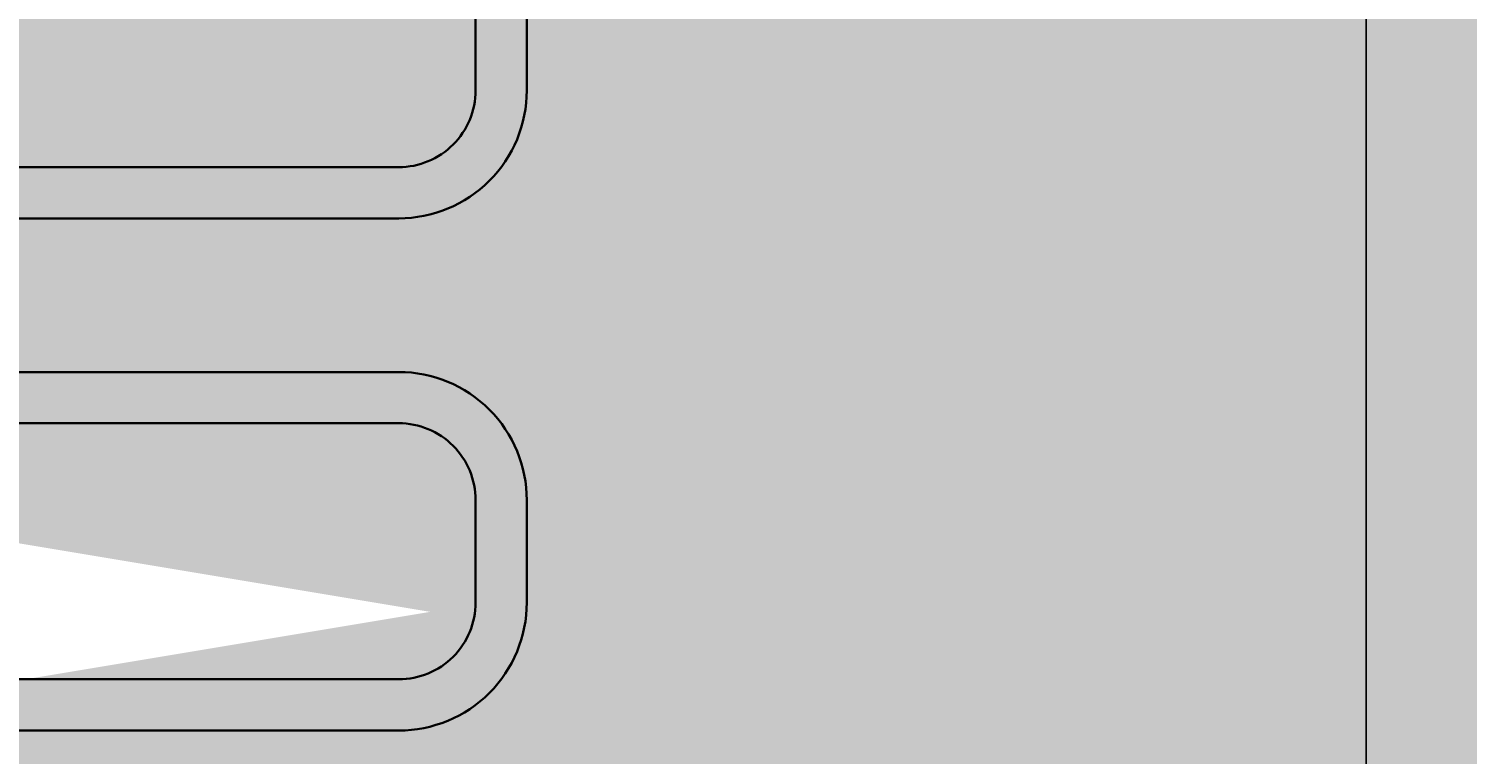
# Model space of a CAD drawing. Units: millimetres. Extents: x -22994 to 29398, y -19990 to 20176.
# Tile 48 of 135: x 170 to 198, y 96 to 110. Entities that reach past the tile are written whole.
import ezdxf

# ---------------------------------------------------------------- set-up
doc = ezdxf.new("R2010")
doc.units = ezdxf.units.MM
doc.header["$MEASUREMENT"] = 0
for name, color, linetype, lineweight in [('M-DIMS', 2, 'Continuous', 18), ('M-EQPM', 7, 'Continuous', 25), ('M-EQPM-PATT', 7, 'Continuous', 18), ('M-PIPE', 7, 'Continuous', 35)]:
    doc.layers.add(name, color=color, linetype=linetype, lineweight=lineweight)
doc.styles.get("Standard").update_dxf_attribs({"font": 'arial.ttf'})
doc.dimstyles.get("Standard").update_dxf_attribs({"dimtxt": 0.18, "dimasz": 10000, "dimexe": 0.18, "dimexo": 0.0625, "dimgap": 0.09, "dimtad": 0, "dimtih": 1, "dimtoh": 1, "dimdec": 0, "dimzin": 0, "dimdsep": 46, "dimtxsty": 'Standard', "dimcen": 0.09, "dimadec": 0, "dimazin": 0, "dimtfac": 1, "dimtdec": 0, "dimtofl": 0, "dimtmove": 0, "dimatfit": 3, "dimfxl": 1, "dimtolj": 1, "dimtzin": 0, "dimlwd": 30, "dimarcsym": 0})

# ---------------------------------------------------------------- blocks, each defined once
blk = doc.blocks.new('*D2')
at = {"layer": 'Defpoints', "color": 0, "transparency": 16777216}
for p in [(6.677, 10.271), (290.852, 10.271), (290.852, -5.079)]:
    blk.add_point(p, dxfattribs=at)
at = {"layer": 'M-DIMS', "color": 0, "lineweight": -2, "transparency": 16777216}
for p, q in [((6.677, 10.209), (6.677, -5.259)), ((290.852, 10.209), (290.852, -5.259))]:
    blk.add_line(p, q, dxfattribs=at)
at = {"layer": 'M-DIMS', "color": 0, "lineweight": 30, "transparency": 16777216}
for p, q in [((-9993.323, -5.079), (-19993.323, -5.079)), ((10290.852, -5.079), (20290.852, -5.079))]:
    blk.add_line(p, q, dxfattribs=at)
at = {"layer": 'M-DIMS', "color": 0, "transparency": 16777216}
for points in [[(-9993.323, 1661.588), (-9993.323, -1671.745), (6.677, -5.079)], [(10290.852, 1661.588), (10290.852, -1671.745), (290.852, -5.079)]]:
    blk.add_solid(points, dxfattribs=at)
at = {"layer": 'M-DIMS', "color": 0, "transparency": 16777216, "insert": (148.765, -5.079), "char_height": 0.18, "attachment_point": 5}
blk.add_mtext('\\A1;284.2', dxfattribs=at)
blk = doc.blocks.new('*D3')
at = {"layer": 'Defpoints', "color": 0, "transparency": 16777216}
for p in [(110.265, 204.165), (110.265, 176.366), (95.833, 127.967)]:
    blk.add_point(p, dxfattribs=at)
at = {"layer": 'M-DIMS', "color": 0, "lineweight": 30, "transparency": 16777216}
for p, q in [((-9904.167, 204.165), (-19904.167, 204.165)), ((10110.265, 204.165), (20110.265, 204.165))]:
    blk.add_line(p, q, dxfattribs=at)
at = {"layer": 'M-DIMS', "color": 0, "lineweight": -2, "transparency": 16777216}
for p, q in [((95.833, 128.03), (95.833, 204.345)), ((110.265, 176.429), (110.265, 204.345))]:
    blk.add_line(p, q, dxfattribs=at)
at = {"layer": 'M-DIMS', "color": 0, "transparency": 16777216}
for points in [[(-9904.167, 1870.832), (-9904.167, -1462.501), (95.833, 204.165)], [(10110.265, 1870.832), (10110.265, -1462.501), (110.265, 204.165)]]:
    blk.add_solid(points, dxfattribs=at)
at = {"layer": 'M-DIMS', "color": 0, "transparency": 16777216, "insert": (103.049, 204.165), "char_height": 0.18, "attachment_point": 5}
blk.add_mtext('\\A1;14.432', dxfattribs=at)
blk = doc.blocks.new('*D4')
at = {"layer": 'Defpoints', "color": 0, "transparency": 16777216}
for p in [(116.265, 204.165), (110.265, 176.366), (116.265, 176.366)]:
    blk.add_point(p, dxfattribs=at)
at = {"layer": 'M-DIMS', "color": 0, "lineweight": 30, "transparency": 16777216}
for p, q in [((-9889.735, 204.165), (-19889.735, 204.165)), ((10116.265, 204.165), (20116.265, 204.165))]:
    blk.add_line(p, q, dxfattribs=at)
at = {"layer": 'M-DIMS', "color": 0, "lineweight": -2, "transparency": 16777216}
for p, q in [((110.265, 176.429), (110.265, 204.345)), ((116.265, 176.429), (116.265, 204.345))]:
    blk.add_line(p, q, dxfattribs=at)
at = {"layer": 'M-DIMS', "color": 0, "transparency": 16777216}
for points in [[(-9889.735, 1870.832), (-9889.735, -1462.501), (110.265, 204.165)], [(10116.265, 1870.832), (10116.265, -1462.501), (116.265, 204.165)]]:
    blk.add_solid(points, dxfattribs=at)
at = {"layer": 'M-DIMS', "color": 0, "transparency": 16777216, "insert": (113.265, 204.165), "char_height": 0.18, "attachment_point": 5}
blk.add_mtext('\\A1;6', dxfattribs=at)
blk = doc.blocks.new('*D5')
at = {"layer": 'Defpoints', "color": 0, "transparency": 16777216}
for p in [(181.265, 204.165), (116.265, 176.366), (181.265, 176.366)]:
    blk.add_point(p, dxfattribs=at)
at = {"layer": 'M-DIMS', "color": 0, "lineweight": 30, "transparency": 16777216}
for p, q in [((-9883.735, 204.165), (-19883.735, 204.165)), ((10181.265, 204.165), (20181.265, 204.165))]:
    blk.add_line(p, q, dxfattribs=at)
at = {"layer": 'M-DIMS', "color": 0, "lineweight": -2, "transparency": 16777216}
for p, q in [((116.265, 176.429), (116.265, 204.345)), ((181.265, 176.429), (181.265, 204.345))]:
    blk.add_line(p, q, dxfattribs=at)
at = {"layer": 'M-DIMS', "color": 0, "transparency": 16777216}
for points in [[(-9883.735, 1870.832), (-9883.735, -1462.501), (116.265, 204.165)], [(10181.265, 1870.832), (10181.265, -1462.501), (181.265, 204.165)]]:
    blk.add_solid(points, dxfattribs=at)
at = {"layer": 'M-DIMS', "color": 0, "transparency": 16777216, "insert": (148.765, 204.165), "char_height": 0.18, "attachment_point": 5}
blk.add_mtext('\\A1;65', dxfattribs=at)
blk = doc.blocks.new('*D6')
at = {"layer": 'Defpoints', "color": 0, "transparency": 16777216}
for p in [(187.265, 204.165), (181.265, 176.366), (187.265, 176.366)]:
    blk.add_point(p, dxfattribs=at)
at = {"layer": 'M-DIMS', "color": 0, "lineweight": 30, "transparency": 16777216}
for p, q in [((-9818.735, 204.165), (-19818.735, 204.165)), ((10187.265, 204.165), (20187.265, 204.165))]:
    blk.add_line(p, q, dxfattribs=at)
at = {"layer": 'M-DIMS', "color": 0, "lineweight": -2, "transparency": 16777216}
for p, q in [((181.265, 176.429), (181.265, 204.345)), ((187.265, 176.429), (187.265, 204.345))]:
    blk.add_line(p, q, dxfattribs=at)
at = {"layer": 'M-DIMS', "color": 0, "transparency": 16777216}
for points in [[(-9818.735, 1870.832), (-9818.735, -1462.501), (181.265, 204.165)], [(10187.265, 1870.832), (10187.265, -1462.501), (187.265, 204.165)]]:
    blk.add_solid(points, dxfattribs=at)
at = {"layer": 'M-DIMS', "color": 0, "transparency": 16777216, "insert": (184.265, 204.165), "char_height": 0.18, "attachment_point": 5}
blk.add_mtext('\\A1;6', dxfattribs=at)
blk = doc.blocks.new('*D7')
at = {"layer": 'Defpoints', "color": 0, "transparency": 16777216}
for p in [(201.697, 204.165), (187.265, 176.366), (201.697, 127.967)]:
    blk.add_point(p, dxfattribs=at)
at = {"layer": 'M-DIMS', "color": 0, "lineweight": 30, "transparency": 16777216}
for p, q in [((-9812.735, 204.165), (-19812.735, 204.165)), ((10201.697, 204.165), (20201.697, 204.165))]:
    blk.add_line(p, q, dxfattribs=at)
at = {"layer": 'M-DIMS', "color": 0, "lineweight": -2, "transparency": 16777216}
for p, q in [((187.265, 176.429), (187.265, 204.345)), ((201.697, 128.03), (201.697, 204.345))]:
    blk.add_line(p, q, dxfattribs=at)
at = {"layer": 'M-DIMS', "color": 0, "transparency": 16777216}
for points in [[(-9812.735, 1870.832), (-9812.735, -1462.501), (187.265, 204.165)], [(10201.697, 1870.832), (10201.697, -1462.501), (201.697, 204.165)]]:
    blk.add_solid(points, dxfattribs=at)
at = {"layer": 'M-DIMS', "color": 0, "transparency": 16777216, "insert": (194.481, 204.165), "char_height": 0.18, "attachment_point": 5}
blk.add_mtext('\\A1;14.432', dxfattribs=at)
blk = doc.blocks.new('*D8')
at = {"layer": 'Defpoints', "color": 0, "transparency": 16777216}
for p in [(227.648, 204.165), (227.648, 146.73), (201.697, 127.967)]:
    blk.add_point(p, dxfattribs=at)
at = {"layer": 'M-DIMS', "color": 0, "lineweight": 30, "transparency": 16777216}
for p, q in [((-9798.303, 204.165), (-19798.303, 204.165)), ((10227.648, 204.165), (20227.648, 204.165))]:
    blk.add_line(p, q, dxfattribs=at)
at = {"layer": 'M-DIMS', "color": 0, "lineweight": -2, "transparency": 16777216}
for p, q in [((201.697, 128.03), (201.697, 204.345)), ((227.648, 146.792), (227.648, 204.345))]:
    blk.add_line(p, q, dxfattribs=at)
at = {"layer": 'M-DIMS', "color": 0, "transparency": 16777216}
for points in [[(-9798.303, 1870.832), (-9798.303, -1462.501), (201.697, 204.165)], [(10227.648, 1870.832), (10227.648, -1462.501), (227.648, 204.165)]]:
    blk.add_solid(points, dxfattribs=at)
at = {"layer": 'M-DIMS', "color": 0, "transparency": 16777216, "insert": (214.673, 204.165), "char_height": 0.18, "attachment_point": 5}
blk.add_mtext('\\A1;25.95', dxfattribs=at)
blk = doc.blocks.new('*D9')
at = {"layer": 'Defpoints', "color": 0, "transparency": 16777216}
for p in [(187.265, 176.366), (306.202, 176.366), (290.852, 10.271)]:
    blk.add_point(p, dxfattribs=at)
at = {"layer": 'M-DIMS', "color": 0, "lineweight": 30, "transparency": 16777216}
for p, q in [((306.202, 10176.366), (306.202, 20176.366)), ((306.202, -9989.729), (306.202, -19989.729))]:
    blk.add_line(p, q, dxfattribs=at)
at = {"layer": 'M-DIMS', "color": 0, "lineweight": -2, "transparency": 16777216}
for p, q in [((187.327, 176.366), (306.382, 176.366)), ((290.915, 10.271), (306.382, 10.271))]:
    blk.add_line(p, q, dxfattribs=at)
at = {"layer": 'M-DIMS', "color": 0, "transparency": 16777216}
for points in [[(-1360.465, 10176.366), (1972.869, 10176.366), (306.202, 176.366)], [(-1360.465, -9989.729), (1972.869, -9989.729), (306.202, 10.271)]]:
    blk.add_solid(points, dxfattribs=at)
at = {"layer": 'M-DIMS', "color": 0, "transparency": 16777216, "insert": (306.202, 93.319), "char_height": 0.18, "attachment_point": 5}
blk.add_mtext('\\A1;166.1', dxfattribs=at)
blk = doc.blocks.new('*D10')
at = {"layer": 'Defpoints', "color": 0, "transparency": 16777216}
for p in [(125.65, 136.071), (133.346, 136.071), (133.346, -5.079)]:
    blk.add_point(p, dxfattribs=at)
at = {"layer": 'M-DIMS', "color": 0, "lineweight": -2, "transparency": 16777216}
for p, q in [((125.65, 136.009), (125.65, -5.259)), ((133.346, 136.009), (133.346, -5.259))]:
    blk.add_line(p, q, dxfattribs=at)
at = {"layer": 'M-DIMS', "color": 0, "lineweight": 30, "transparency": 16777216}
for p, q in [((-9874.35, -5.079), (-19874.35, -5.079)), ((10133.346, -5.079), (20133.346, -5.079))]:
    blk.add_line(p, q, dxfattribs=at)
at = {"layer": 'M-DIMS', "color": 0, "transparency": 16777216}
for points in [[(-9874.35, 1661.588), (-9874.35, -1671.745), (125.65, -5.079)], [(10133.346, 1661.588), (10133.346, -1671.745), (133.346, -5.079)]]:
    blk.add_solid(points, dxfattribs=at)
at = {"layer": 'M-DIMS', "color": 0, "transparency": 16777216, "insert": (129.498, -5.079), "char_height": 0.18, "attachment_point": 5}
blk.add_mtext('\\A1;7.696', dxfattribs=at)
blk = doc.blocks.new('*D11')
at = {"layer": 'Defpoints', "color": 0, "transparency": 16777216}
for p in [(133.346, 136.071), (135.65, 136.071), (135.65, -5.079)]:
    blk.add_point(p, dxfattribs=at)
at = {"layer": 'M-DIMS', "color": 0, "lineweight": -2, "transparency": 16777216}
for p, q in [((133.346, 136.009), (133.346, -5.259)), ((135.65, 136.009), (135.65, -5.259))]:
    blk.add_line(p, q, dxfattribs=at)
at = {"layer": 'M-DIMS', "color": 0, "lineweight": 30, "transparency": 16777216}
for p, q in [((-9866.654, -5.079), (-19866.654, -5.079)), ((10135.65, -5.079), (20135.65, -5.079))]:
    blk.add_line(p, q, dxfattribs=at)
at = {"layer": 'M-DIMS', "color": 0, "transparency": 16777216}
for points in [[(-9866.654, 1661.588), (-9866.654, -1671.745), (133.346, -5.079)], [(10135.65, 1661.588), (10135.65, -1671.745), (135.65, -5.079)]]:
    blk.add_solid(points, dxfattribs=at)
at = {"layer": 'M-DIMS', "color": 0, "transparency": 16777216, "insert": (134.498, -5.079), "char_height": 0.18, "attachment_point": 5}
blk.add_mtext('\\A1;2.304', dxfattribs=at)
blk = doc.blocks.new('*D12')
at = {"layer": 'Defpoints', "color": 0, "transparency": 16777216}
for p in [(135.65, 136.071), (145.65, 136.071), (145.65, -5.079)]:
    blk.add_point(p, dxfattribs=at)
at = {"layer": 'M-DIMS', "color": 0, "lineweight": -2, "transparency": 16777216}
for p, q in [((135.65, 136.009), (135.65, -5.259)), ((145.65, 136.009), (145.65, -5.259))]:
    blk.add_line(p, q, dxfattribs=at)
at = {"layer": 'M-DIMS', "color": 0, "lineweight": 30, "transparency": 16777216}
for p, q in [((-9864.35, -5.079), (-19864.35, -5.079)), ((10145.65, -5.079), (20145.65, -5.079))]:
    blk.add_line(p, q, dxfattribs=at)
at = {"layer": 'M-DIMS', "color": 0, "transparency": 16777216}
for points in [[(-9864.35, 1661.588), (-9864.35, -1671.745), (135.65, -5.079)], [(10145.65, 1661.588), (10145.65, -1671.745), (145.65, -5.079)]]:
    blk.add_solid(points, dxfattribs=at)
at = {"layer": 'M-DIMS', "color": 0, "transparency": 16777216, "insert": (140.65, -5.079), "char_height": 0.18, "attachment_point": 5}
blk.add_mtext('\\A1;10', dxfattribs=at)
blk = doc.blocks.new('*D13')
at = {"layer": 'Defpoints', "color": 0, "transparency": 16777216}
for p in [(145.65, 136.071), (155.65, 136.071), (155.65, -5.079)]:
    blk.add_point(p, dxfattribs=at)
at = {"layer": 'M-DIMS', "color": 0, "lineweight": -2, "transparency": 16777216}
for p, q in [((145.65, 136.009), (145.65, -5.259)), ((155.65, 136.009), (155.65, -5.259))]:
    blk.add_line(p, q, dxfattribs=at)
at = {"layer": 'M-DIMS', "color": 0, "lineweight": 30, "transparency": 16777216}
for p, q in [((-9854.35, -5.079), (-19854.35, -5.079)), ((10155.65, -5.079), (20155.65, -5.079))]:
    blk.add_line(p, q, dxfattribs=at)
at = {"layer": 'M-DIMS', "color": 0, "transparency": 16777216}
for points in [[(-9854.35, 1661.588), (-9854.35, -1671.745), (145.65, -5.079)], [(10155.65, 1661.588), (10155.65, -1671.745), (155.65, -5.079)]]:
    blk.add_solid(points, dxfattribs=at)
at = {"layer": 'M-DIMS', "color": 0, "transparency": 16777216, "insert": (150.65, -5.079), "char_height": 0.18, "attachment_point": 5}
blk.add_mtext('\\A1;10', dxfattribs=at)
blk = doc.blocks.new('*D14')
at = {"layer": 'Defpoints', "color": 0, "transparency": 16777216}
for p in [(155.65, 136.071), (165.65, 136.071), (165.65, -5.079)]:
    blk.add_point(p, dxfattribs=at)
at = {"layer": 'M-DIMS', "color": 0, "lineweight": -2, "transparency": 16777216}
for p, q in [((155.65, 136.009), (155.65, -5.259)), ((165.65, 136.009), (165.65, -5.259))]:
    blk.add_line(p, q, dxfattribs=at)
at = {"layer": 'M-DIMS', "color": 0, "lineweight": 30, "transparency": 16777216}
for p, q in [((-9844.35, -5.079), (-19844.35, -5.079)), ((10165.65, -5.079), (20165.65, -5.079))]:
    blk.add_line(p, q, dxfattribs=at)
at = {"layer": 'M-DIMS', "color": 0, "transparency": 16777216}
for points in [[(-9844.35, 1661.588), (-9844.35, -1671.745), (155.65, -5.079)], [(10165.65, 1661.588), (10165.65, -1671.745), (165.65, -5.079)]]:
    blk.add_solid(points, dxfattribs=at)
at = {"layer": 'M-DIMS', "color": 0, "transparency": 16777216, "insert": (160.65, -5.079), "char_height": 0.18, "attachment_point": 5}
blk.add_mtext('\\A1;10', dxfattribs=at)
blk = doc.blocks.new('*D15')
at = {"layer": 'Defpoints', "color": 0, "transparency": 16777216}
for p in [(173.346, 154.788), (173.346, 136.071), (306.202, 136.071)]:
    blk.add_point(p, dxfattribs=at)
at = {"layer": 'M-DIMS', "color": 0, "lineweight": 30, "transparency": 16777216}
for p, q in [((306.202, 10154.788), (306.202, 20154.788)), ((306.202, -9863.929), (306.202, -19863.929))]:
    blk.add_line(p, q, dxfattribs=at)
at = {"layer": 'M-DIMS', "color": 0, "lineweight": -2, "transparency": 16777216}
for p, q in [((173.408, 154.788), (306.382, 154.788)), ((173.408, 136.071), (306.382, 136.071))]:
    blk.add_line(p, q, dxfattribs=at)
at = {"layer": 'M-DIMS', "color": 0, "transparency": 16777216}
for points in [[(-1360.465, 10154.788), (1972.869, 10154.788), (306.202, 154.788)], [(-1360.465, -9863.929), (1972.869, -9863.929), (306.202, 136.071)]]:
    blk.add_solid(points, dxfattribs=at)
at = {"layer": 'M-DIMS', "color": 0, "transparency": 16777216, "insert": (306.202, 145.43), "char_height": 0.18, "attachment_point": 5}
blk.add_mtext('\\A1;18.717', dxfattribs=at)
blk = doc.blocks.new('*D16')
at = {"layer": 'Defpoints', "color": 0, "transparency": 16777216}
for p in [(120.17, 204.165), (110.466, 48.035), (120.17, 48.035)]:
    blk.add_point(p, dxfattribs=at)
at = {"layer": 'M-DIMS', "color": 0, "lineweight": 30, "transparency": 16777216}
for p, q in [((-9889.534, 204.165), (-19889.534, 204.165)), ((10120.17, 204.165), (20120.17, 204.165))]:
    blk.add_line(p, q, dxfattribs=at)
at = {"layer": 'M-DIMS', "color": 0, "lineweight": -2, "transparency": 16777216}
for p, q in [((110.466, 48.097), (110.466, 204.345)), ((120.17, 48.097), (120.17, 204.345))]:
    blk.add_line(p, q, dxfattribs=at)
at = {"layer": 'M-DIMS', "color": 0, "transparency": 16777216}
for points in [[(-9889.534, 1870.832), (-9889.534, -1462.501), (110.466, 204.165)], [(10120.17, 1870.832), (10120.17, -1462.501), (120.17, 204.165)]]:
    blk.add_solid(points, dxfattribs=at)
at = {"layer": 'M-DIMS', "color": 0, "transparency": 16777216, "insert": (115.318, 204.165), "char_height": 0.18, "attachment_point": 5}
blk.add_mtext('\\A1;9.704', dxfattribs=at)
blk = doc.blocks.new('*D17')
at = {"layer": 'Defpoints', "color": 0, "transparency": 16777216}
for p in [(126.17, 204.165), (120.17, 48.035), (126.17, 48.035)]:
    blk.add_point(p, dxfattribs=at)
at = {"layer": 'M-DIMS', "color": 0, "lineweight": 30, "transparency": 16777216}
for p, q in [((-9879.83, 204.165), (-19879.83, 204.165)), ((10126.17, 204.165), (20126.17, 204.165))]:
    blk.add_line(p, q, dxfattribs=at)
at = {"layer": 'M-DIMS', "color": 0, "lineweight": -2, "transparency": 16777216}
for p, q in [((120.17, 48.097), (120.17, 204.345)), ((126.17, 48.097), (126.17, 204.345))]:
    blk.add_line(p, q, dxfattribs=at)
at = {"layer": 'M-DIMS', "color": 0, "transparency": 16777216}
for points in [[(-9879.83, 1870.832), (-9879.83, -1462.501), (120.17, 204.165)], [(10126.17, 1870.832), (10126.17, -1462.501), (126.17, 204.165)]]:
    blk.add_solid(points, dxfattribs=at)
at = {"layer": 'M-DIMS', "color": 0, "transparency": 16777216, "insert": (123.17, 204.165), "char_height": 0.18, "attachment_point": 5}
blk.add_mtext('\\A1;6', dxfattribs=at)
blk = doc.blocks.new('*D18')
at = {"layer": 'Defpoints', "color": 0, "transparency": 16777216}
for p in [(132.17, 204.165), (126.17, 48.035), (132.17, 48.035)]:
    blk.add_point(p, dxfattribs=at)
at = {"layer": 'M-DIMS', "color": 0, "lineweight": 30, "transparency": 16777216}
for p, q in [((-9873.83, 204.165), (-19873.83, 204.165)), ((10132.17, 204.165), (20132.17, 204.165))]:
    blk.add_line(p, q, dxfattribs=at)
at = {"layer": 'M-DIMS', "color": 0, "lineweight": -2, "transparency": 16777216}
for p, q in [((126.17, 48.097), (126.17, 204.345)), ((132.17, 48.097), (132.17, 204.345))]:
    blk.add_line(p, q, dxfattribs=at)
at = {"layer": 'M-DIMS', "color": 0, "transparency": 16777216}
for points in [[(-9873.83, 1870.832), (-9873.83, -1462.501), (126.17, 204.165)], [(10132.17, 1870.832), (10132.17, -1462.501), (132.17, 204.165)]]:
    blk.add_solid(points, dxfattribs=at)
at = {"layer": 'M-DIMS', "color": 0, "transparency": 16777216, "insert": (129.17, 204.165), "char_height": 0.18, "attachment_point": 5}
blk.add_mtext('\\A1;6', dxfattribs=at)
blk = doc.blocks.new('*D19')
at = {"layer": 'Defpoints', "color": 0, "transparency": 16777216}
for p in [(138.17, 204.165), (132.17, 48.035), (138.17, 48.035)]:
    blk.add_point(p, dxfattribs=at)
at = {"layer": 'M-DIMS', "color": 0, "lineweight": 30, "transparency": 16777216}
for p, q in [((-9867.83, 204.165), (-19867.83, 204.165)), ((10138.17, 204.165), (20138.17, 204.165))]:
    blk.add_line(p, q, dxfattribs=at)
at = {"layer": 'M-DIMS', "color": 0, "lineweight": -2, "transparency": 16777216}
for p, q in [((132.17, 48.097), (132.17, 204.345)), ((138.17, 48.097), (138.17, 204.345))]:
    blk.add_line(p, q, dxfattribs=at)
at = {"layer": 'M-DIMS', "color": 0, "transparency": 16777216}
for points in [[(-9867.83, 1870.832), (-9867.83, -1462.501), (132.17, 204.165)], [(10138.17, 1870.832), (10138.17, -1462.501), (138.17, 204.165)]]:
    blk.add_solid(points, dxfattribs=at)
at = {"layer": 'M-DIMS', "color": 0, "transparency": 16777216, "insert": (135.17, 204.165), "char_height": 0.18, "attachment_point": 5}
blk.add_mtext('\\A1;6', dxfattribs=at)
blk = doc.blocks.new('*D20')
at = {"layer": 'Defpoints', "color": 0, "transparency": 16777216}
for p in [(144.17, 204.165), (138.17, 48.035), (144.17, 48.035)]:
    blk.add_point(p, dxfattribs=at)
at = {"layer": 'M-DIMS', "color": 0, "lineweight": 30, "transparency": 16777216}
for p, q in [((-9861.83, 204.165), (-19861.83, 204.165)), ((10144.17, 204.165), (20144.17, 204.165))]:
    blk.add_line(p, q, dxfattribs=at)
at = {"layer": 'M-DIMS', "color": 0, "lineweight": -2, "transparency": 16777216}
for p, q in [((138.17, 48.097), (138.17, 204.345)), ((144.17, 48.097), (144.17, 204.345))]:
    blk.add_line(p, q, dxfattribs=at)
at = {"layer": 'M-DIMS', "color": 0, "transparency": 16777216}
for points in [[(-9861.83, 1870.832), (-9861.83, -1462.501), (138.17, 204.165)], [(10144.17, 1870.832), (10144.17, -1462.501), (144.17, 204.165)]]:
    blk.add_solid(points, dxfattribs=at)
at = {"layer": 'M-DIMS', "color": 0, "transparency": 16777216, "insert": (141.17, 204.165), "char_height": 0.18, "attachment_point": 5}
blk.add_mtext('\\A1;6', dxfattribs=at)
blk = doc.blocks.new('*D21')
at = {"layer": 'Defpoints', "color": 0, "transparency": 16777216}
for p in [(149.116, 204.165), (144.17, 48.035), (149.116, 48.035)]:
    blk.add_point(p, dxfattribs=at)
at = {"layer": 'M-DIMS', "color": 0, "lineweight": 30, "transparency": 16777216}
for p, q in [((-9855.83, 204.165), (-19855.83, 204.165)), ((10149.116, 204.165), (20149.116, 204.165))]:
    blk.add_line(p, q, dxfattribs=at)
at = {"layer": 'M-DIMS', "color": 0, "lineweight": -2, "transparency": 16777216}
for p, q in [((144.17, 48.097), (144.17, 204.345)), ((149.116, 48.097), (149.116, 204.345))]:
    blk.add_line(p, q, dxfattribs=at)
at = {"layer": 'M-DIMS', "color": 0, "transparency": 16777216}
for points in [[(-9855.83, 1870.832), (-9855.83, -1462.501), (144.17, 204.165)], [(10149.116, 1870.832), (10149.116, -1462.501), (149.116, 204.165)]]:
    blk.add_solid(points, dxfattribs=at)
at = {"layer": 'M-DIMS', "color": 0, "transparency": 16777216, "insert": (146.643, 204.165), "char_height": 0.18, "attachment_point": 5}
blk.add_mtext('\\A1;4.945', dxfattribs=at)
blk = doc.blocks.new('*D22')
at = {"layer": 'Defpoints', "color": 0, "transparency": 16777216}
for p in [(149.116, 30.99), (155.116, 30.99), (155.116, -5.079)]:
    blk.add_point(p, dxfattribs=at)
at = {"layer": 'M-DIMS', "color": 0, "lineweight": -2, "transparency": 16777216}
for p, q in [((149.116, 30.927), (149.116, -5.259)), ((155.116, 30.927), (155.116, -5.259))]:
    blk.add_line(p, q, dxfattribs=at)
at = {"layer": 'M-DIMS', "color": 0, "lineweight": 30, "transparency": 16777216}
for p, q in [((-9850.884, -5.079), (-19850.884, -5.079)), ((10155.116, -5.079), (20155.116, -5.079))]:
    blk.add_line(p, q, dxfattribs=at)
at = {"layer": 'M-DIMS', "color": 0, "transparency": 16777216}
for points in [[(-9850.884, 1661.588), (-9850.884, -1671.745), (149.116, -5.079)], [(10155.116, 1661.588), (10155.116, -1671.745), (155.116, -5.079)]]:
    blk.add_solid(points, dxfattribs=at)
at = {"layer": 'M-DIMS', "color": 0, "transparency": 16777216, "insert": (152.116, -5.079), "char_height": 0.18, "attachment_point": 5}
blk.add_mtext('\\A1;6', dxfattribs=at)
blk = doc.blocks.new('*D23')
at = {"layer": 'Defpoints', "color": 0, "transparency": 16777216}
for p in [(155.116, 30.99), (161.116, 30.99), (161.116, -5.079)]:
    blk.add_point(p, dxfattribs=at)
at = {"layer": 'M-DIMS', "color": 0, "lineweight": -2, "transparency": 16777216}
for p, q in [((155.116, 30.927), (155.116, -5.259)), ((161.116, 30.927), (161.116, -5.259))]:
    blk.add_line(p, q, dxfattribs=at)
at = {"layer": 'M-DIMS', "color": 0, "lineweight": 30, "transparency": 16777216}
for p, q in [((-9844.884, -5.079), (-19844.884, -5.079)), ((10161.116, -5.079), (20161.116, -5.079))]:
    blk.add_line(p, q, dxfattribs=at)
at = {"layer": 'M-DIMS', "color": 0, "transparency": 16777216}
for points in [[(-9844.884, 1661.588), (-9844.884, -1671.745), (155.116, -5.079)], [(10161.116, 1661.588), (10161.116, -1671.745), (161.116, -5.079)]]:
    blk.add_solid(points, dxfattribs=at)
at = {"layer": 'M-DIMS', "color": 0, "transparency": 16777216, "insert": (158.116, -5.079), "char_height": 0.18, "attachment_point": 5}
blk.add_mtext('\\A1;6', dxfattribs=at)
blk = doc.blocks.new('*D24')
at = {"layer": 'Defpoints', "color": 0, "transparency": 16777216}
for p in [(161.116, 30.99), (166.439, 30.99), (166.439, -5.079)]:
    blk.add_point(p, dxfattribs=at)
at = {"layer": 'M-DIMS', "color": 0, "lineweight": -2, "transparency": 16777216}
for p, q in [((161.116, 30.927), (161.116, -5.259)), ((166.439, 30.927), (166.439, -5.259))]:
    blk.add_line(p, q, dxfattribs=at)
at = {"layer": 'M-DIMS', "color": 0, "lineweight": 30, "transparency": 16777216}
for p, q in [((-9838.884, -5.079), (-19838.884, -5.079)), ((10166.439, -5.079), (20166.439, -5.079))]:
    blk.add_line(p, q, dxfattribs=at)
at = {"layer": 'M-DIMS', "color": 0, "transparency": 16777216}
for points in [[(-9838.884, 1661.588), (-9838.884, -1671.745), (161.116, -5.079)], [(10166.439, 1661.588), (10166.439, -1671.745), (166.439, -5.079)]]:
    blk.add_solid(points, dxfattribs=at)
at = {"layer": 'M-DIMS', "color": 0, "transparency": 16777216, "insert": (163.777, -5.079), "char_height": 0.18, "attachment_point": 5}
blk.add_mtext('\\A1;5.323', dxfattribs=at)
blk = doc.blocks.new('*D25')
at = {"layer": 'Defpoints', "color": 0, "transparency": 16777216}
for p in [(166.439, 30.99), (172.439, 30.99), (172.439, -5.079)]:
    blk.add_point(p, dxfattribs=at)
at = {"layer": 'M-DIMS', "color": 0, "lineweight": -2, "transparency": 16777216}
for p, q in [((166.439, 30.927), (166.439, -5.259)), ((172.439, 30.927), (172.439, -5.259))]:
    blk.add_line(p, q, dxfattribs=at)
at = {"layer": 'M-DIMS', "color": 0, "lineweight": 30, "transparency": 16777216}
for p, q in [((-9833.561, -5.079), (-19833.561, -5.079)), ((10172.439, -5.079), (20172.439, -5.079))]:
    blk.add_line(p, q, dxfattribs=at)
at = {"layer": 'M-DIMS', "color": 0, "transparency": 16777216}
for points in [[(-9833.561, 1661.588), (-9833.561, -1671.745), (166.439, -5.079)], [(10172.439, 1661.588), (10172.439, -1671.745), (172.439, -5.079)]]:
    blk.add_solid(points, dxfattribs=at)
at = {"layer": 'M-DIMS', "color": 0, "transparency": 16777216, "insert": (169.439, -5.079), "char_height": 0.18, "attachment_point": 5}
blk.add_mtext('\\A1;6', dxfattribs=at)
blk = doc.blocks.new('*D26')
at = {"layer": 'Defpoints', "color": 0, "transparency": 16777216}
for p in [(172.439, 30.99), (178.439, 30.99), (178.439, -5.079)]:
    blk.add_point(p, dxfattribs=at)
at = {"layer": 'M-DIMS', "color": 0, "lineweight": -2, "transparency": 16777216}
for p, q in [((172.439, 30.927), (172.439, -5.259)), ((178.439, 30.927), (178.439, -5.259))]:
    blk.add_line(p, q, dxfattribs=at)
at = {"layer": 'M-DIMS', "color": 0, "lineweight": 30, "transparency": 16777216}
for p, q in [((-9827.561, -5.079), (-19827.561, -5.079)), ((10178.439, -5.079), (20178.439, -5.079))]:
    blk.add_line(p, q, dxfattribs=at)
at = {"layer": 'M-DIMS', "color": 0, "transparency": 16777216}
for points in [[(-9827.561, 1661.588), (-9827.561, -1671.745), (172.439, -5.079)], [(10178.439, 1661.588), (10178.439, -1671.745), (178.439, -5.079)]]:
    blk.add_solid(points, dxfattribs=at)
at = {"layer": 'M-DIMS', "color": 0, "transparency": 16777216, "insert": (175.439, -5.079), "char_height": 0.18, "attachment_point": 5}
blk.add_mtext('\\A1;6', dxfattribs=at)
blk = doc.blocks.new('*D27')
at = {"layer": 'Defpoints', "color": 0, "transparency": 16777216}
for p in [(178.439, 30.99), (188.117, 30.99), (188.117, -5.079)]:
    blk.add_point(p, dxfattribs=at)
at = {"layer": 'M-DIMS', "color": 0, "lineweight": -2, "transparency": 16777216}
for p, q in [((178.439, 30.927), (178.439, -5.259)), ((188.117, 30.927), (188.117, -5.259))]:
    blk.add_line(p, q, dxfattribs=at)
at = {"layer": 'M-DIMS', "color": 0, "lineweight": 30, "transparency": 16777216}
for p, q in [((-9821.561, -5.079), (-19821.561, -5.079)), ((10188.117, -5.079), (20188.117, -5.079))]:
    blk.add_line(p, q, dxfattribs=at)
at = {"layer": 'M-DIMS', "color": 0, "transparency": 16777216}
for points in [[(-9821.561, 1661.588), (-9821.561, -1671.745), (178.439, -5.079)], [(10188.117, 1661.588), (10188.117, -1671.745), (188.117, -5.079)]]:
    blk.add_solid(points, dxfattribs=at)
at = {"layer": 'M-DIMS', "color": 0, "transparency": 16777216, "insert": (183.278, -5.079), "char_height": 0.18, "attachment_point": 5}
blk.add_mtext('\\A1;9.679', dxfattribs=at)
blk = doc.blocks.new('*D28')
at = {"layer": 'Defpoints', "color": 0, "transparency": 16777216}
for p in [(188.117, 48.035), (306.202, 48.035), (188.117, 30.99)]:
    blk.add_point(p, dxfattribs=at)
at = {"layer": 'M-DIMS', "color": 0, "lineweight": 30, "transparency": 16777216}
for p, q in [((306.202, 10048.035), (306.202, 20048.035)), ((306.202, -9969.01), (306.202, -19969.01))]:
    blk.add_line(p, q, dxfattribs=at)
at = {"layer": 'M-DIMS', "color": 0, "lineweight": -2, "transparency": 16777216}
for p, q in [((188.18, 48.035), (306.382, 48.035)), ((188.18, 30.99), (306.382, 30.99))]:
    blk.add_line(p, q, dxfattribs=at)
at = {"layer": 'M-DIMS', "color": 0, "transparency": 16777216}
for points in [[(-1360.465, 10048.035), (1972.869, 10048.035), (306.202, 48.035)], [(-1360.465, -9969.01), (1972.869, -9969.01), (306.202, 30.99)]]:
    blk.add_solid(points, dxfattribs=at)
at = {"layer": 'M-DIMS', "color": 0, "transparency": 16777216, "insert": (306.202, 39.512), "char_height": 0.18, "attachment_point": 5}
blk.add_mtext('\\A1;17.045', dxfattribs=at)
blk = doc.blocks.new('*D29')
at = {"layer": 'Defpoints', "color": 0, "transparency": 16777216}
for p in [(36.801, 80.045), (64.03, 80.045)]:
    blk.add_point(p, dxfattribs=at)
at = {"layer": 'M-DIMS', "color": 0, "lineweight": -2, "transparency": 16777216}
for p, q in [((50.325, 80.045), (50.505, 80.045)), ((50.415, 79.955), (50.415, 80.135))]:
    blk.add_line(p, q, dxfattribs=at)
at = {"layer": 'M-DIMS', "color": 0, "lineweight": 30, "transparency": 16777216}
blk.add_line((20064.03, 80.03), (10064.03, 80.038), dxfattribs=at)
at = {"layer": 'M-DIMS', "color": 0, "transparency": 16777216}
blk.add_solid([(10064.031, 1746.704), (10064.028, -1586.629), (64.03, 80.045)], dxfattribs=at)
at = {"layer": 'M-DIMS', "color": 0, "transparency": 16777216, "insert": (20064.521, 80.03), "char_height": 0.18, "attachment_point": 5}
blk.add_mtext('\\A1;∅27.23', dxfattribs=at)
blk = doc.blocks.new('*D36')
at = {"layer": 'Defpoints', "color": 0, "transparency": 16777216}
for p in [(46.39, 31.303), (46.387, 26.593)]:
    blk.add_point(p, dxfattribs=at)
at = {"layer": 'M-DIMS', "color": 0, "lineweight": 30, "transparency": 16777216}
for p, q in [((57.15, 20031.301), (51.77, 10031.302)), ((10057.15, 20031.301), (57.15, 20031.301))]:
    blk.add_line(p, q, dxfattribs=at)
at = {"layer": 'M-DIMS', "color": 0, "lineweight": -2, "transparency": 16777216}
for p, q in [((46.299, 28.948), (46.479, 28.948)), ((46.389, 28.858), (46.389, 29.038))]:
    blk.add_line(p, q, dxfattribs=at)
at = {"layer": 'M-DIMS', "color": 0, "transparency": 16777216}
blk.add_solid([(-1614.896, 10032.199), (1718.436, 10030.405), (46.39, 31.303)], dxfattribs=at)
at = {"layer": 'M-DIMS', "color": 0, "transparency": 16777216, "insert": (10057.554, 20031.301), "char_height": 0.18, "attachment_point": 5}
blk.add_mtext('\\A1;∅4.71', dxfattribs=at)
blk = doc.blocks.new('*D37')
at = {"layer": 'Defpoints', "color": 0, "transparency": 16777216}
for p in [(54.834, 118.615), (59.494, 118.614)]:
    blk.add_point(p, dxfattribs=at)
at = {"layer": 'M-DIMS', "color": 0, "lineweight": -2, "transparency": 16777216}
for p, q in [((57.074, 118.614), (57.254, 118.614)), ((57.164, 118.524), (57.164, 118.704))]:
    blk.add_line(p, q, dxfattribs=at)
at = {"layer": 'M-DIMS', "color": 0, "lineweight": 30, "transparency": 16777216}
blk.add_line((20059.493, 116.253), (10059.494, 117.434), dxfattribs=at)
at = {"layer": 'M-DIMS', "color": 0, "transparency": 16777216}
blk.add_solid([(10059.69, 1784.1), (10059.297, -1549.233), (59.494, 118.614)], dxfattribs=at)
at = {"layer": 'M-DIMS', "color": 0, "transparency": 16777216, "insert": (20059.985, 116.253), "char_height": 0.18, "attachment_point": 5}
blk.add_mtext('\\A1;∅4.659', dxfattribs=at)

msp = doc.modelspace()

# ---------------------------------------------------------------- hatches: boundary and pattern name
at = {"layer": 'M-EQPM-PATT'}
h = msp.add_hatch(color=256, dxfattribs=at)
h.set_gradient(color1=(205, 32, 39), color2=(205, 32, 39), tint=1)
h.paths.add_polyline_path([(116.2647, 150.3662), (116.2647, 170.3662), (116.2647, 176.3662), (110.2647, 176.3662), (110.2647, 152.0276), (95.8327, 127.967), (95.8327, 16.6063), (201.6967, 16.6063), (201.6967, 127.967), (187.2647, 152.0276), (187.2647, 176.3662), (181.2647, 176.3662), (181.2647, 170.3662), (181.2647, 150.3662), (195.6967, 126.3055), (195.6967, 22.6063), (101.8327, 22.6063), (101.8327, 126.3055)])
h.paths.add_polyline_path([(185.2208, 88.6347), (101.8327, 88.6347), (101.8327, 87.6347), (182.8066, 87.6347), (178.7313, 83.5594), (195.6967, 83.5594), (195.6967, 84.5594), (181.1455, 84.5594)], flags=17)
h.paths.add_polyline_path([(95.8327, 88.6347), (60.9779, 88.6347, -0.0228552), (61.7178, 87.6347), (95.8327, 87.6347)])
h.paths.add_polyline_path([(215.6212, 86.5189), (215.6212, 80.5999), (220.5095, 83.5594)])
h.paths.add_polyline_path([(215.6212, 84.5594), (201.6967, 84.5594), (201.6967, 83.5594), (215.6212, 83.5594)])
h.paths.add_polyline_path([(225.3978, 86.5189), (220.5095, 83.5594), (225.3978, 80.5999)])
h.paths.add_polyline_path([(231.6256, 84.5594), (225.3978, 84.5594), (225.3978, 83.5594), (231.6256, 83.5594)])
h = msp.add_hatch(color=256, dxfattribs=at)
h.set_gradient(color1=(34, 52, 110), color2=(41, 49, 137), tint=1, name='CYLINDER')
h.paths.add_polyline_path([(101.8327, 123.6277), (101.8327, 122.6277), (176.8123, 122.6277, -0.4142136), (178.3123, 121.1277), (178.3123, 119.1277, -0.4142136), (176.8123, 117.6277), (129.8123, 117.6277, 0.4142136), (128.3123, 116.1277), (128.3123, 114.1277, 0.4142136), (129.8123, 112.6277), (176.8123, 112.6277, -0.4142136), (178.3123, 111.1277), (178.3123, 109.1277, -0.4142136), (176.8123, 107.6277), (129.8123, 107.6277, 0.4142136), (128.3123, 106.1277), (128.3123, 104.1277, 0.4142136), (129.8123, 102.6277), (176.8123, 102.6277, -0.4142136), (178.3123, 101.1277), (178.3123, 99.1277, -0.4142136), (176.8123, 97.6277), (101.8327, 97.6277), (101.8327, 96.6277), (176.8123, 96.6277, 0.4142136), (179.3123, 99.1277), (179.3123, 101.1277, 0.4142136), (176.8123, 103.6277), (129.8123, 103.6277, -0.4142136), (129.3123, 104.1277), (129.3123, 106.1277, -0.4142136), (129.8123, 106.6277), (176.8123, 106.6277, 0.4142136), (179.3123, 109.1277), (179.3123, 111.1277, 0.4142136), (176.8123, 113.6277), (129.8123, 113.6277, -0.4142136), (129.3123, 114.1277), (129.3123, 116.1277, -0.4142136), (129.8123, 116.6277), (176.8123, 116.6277, 0.4142136), (179.3123, 119.1277), (179.3123, 121.1277, 0.4142136), (176.8123, 123.6277)])
h.paths.add_polyline_path([(75.6657, 123.6277), (75.6657, 122.6277), (95.8327, 122.6277), (95.8327, 123.6277)])
h.paths.add_polyline_path([(51.0853, 122.6277, -0.0439182), (51.8797, 123.6277), (38.9157, 123.6277), (38.9157, 122.6277)])
h.paths.add_polyline_path([(95.8327, 96.6277), (95.8327, 97.6277), (22.2694, 97.6277, 0.4142136), (20.7694, 96.1277), (20.7694, 89.8712, 0.4142136), (22.2694, 88.3712), (39.6435, 88.3712, -0.024152), (40.4967, 89.3712), (23.2694, 89.3712, -0.4142136), (21.7694, 90.8712), (21.7694, 95.1277, -0.4142136), (23.2694, 96.6277)])
h.paths.add_polyline_path([(137.7248, 106.4435), (168.6853, 106.4435), (168.6853, 114.6864), (137.7248, 114.6864)], flags=25)

# ---------------------------------------------------------------- linework, layer by layer
at = {"layer": 'M-EQPM'}
msp.add_lwpolyline([(116.2647, 170.3662), (116.2647, 150.3662), (101.8327, 126.3055), (101.8327, 22.6063), (195.6967, 22.6063), (195.6967, 126.3055), (181.2647, 150.3662), (181.2647, 170.3662)], dxfattribs=at)
at = {"layer": 'M-PIPE'}
for points in [[(101.8327, 123.6277), (176.8123, 123.6277, -0.4142136), (179.3123, 121.1277), (179.3123, 119.1277, -0.4142136), (176.8123, 116.6277), (129.8123, 116.6277, 0.4142136), (129.3123, 116.1277), (129.3123, 114.1277, 0.4142136), (129.8123, 113.6277), (176.8123, 113.6277, -0.4142136), (179.3123, 111.1277), (179.3123, 109.1277, -0.4142136), (176.8123, 106.6277), (129.8123, 106.6277, 0.4142136), (129.3123, 106.1277), (129.3123, 104.1277, 0.4142136), (129.8123, 103.6277), (176.8123, 103.6277, -0.4142136), (179.3123, 101.1277), (179.3123, 99.1277, -0.4142136), (176.8123, 96.6277), (101.8327, 96.6277)], [(101.8327, 122.6277), (176.8123, 122.6277, -0.4142136), (178.3123, 121.1277), (178.3123, 119.1277, -0.4142136), (176.8123, 117.6277), (129.8123, 117.6277, 0.4142136), (128.3123, 116.1277), (128.3123, 114.1277, 0.4142136), (129.8123, 112.6277), (176.8123, 112.6277, -0.4142136), (178.3123, 111.1277), (178.3123, 109.1277, -0.4142136), (176.8123, 107.6277), (129.8123, 107.6277, 0.4142136), (128.3123, 106.1277), (128.3123, 104.1277, 0.4142136), (129.8123, 102.6277), (176.8123, 102.6277, -0.4142136), (178.3123, 101.1277), (178.3123, 99.1277, -0.4142136), (176.8123, 97.6277), (101.8327, 97.6277)]]:
    msp.add_lwpolyline(points, format="xyb", dxfattribs=at)

# ---------------------------------------------------------------- dimensions: what is measured, and where the dimension line sits
at = {"layer": 'M-DIMS'}
for base, p1, p2, override, picture, middle in [((306.202, 176.3662), (290.852, 10.2713), (187.2647, 176.3662), {"dimdec": 1, "dimlfac": 1, "dimrnd": 0, "dimzin": 0, "dimdsep": 46, "dimlunit": 2}, '*D9', (306.202, 93.3187)), ((306.202, 136.0713), (173.3459, 154.788), (173.3459, 136.0713), {"dimdec": 3, "dimlfac": 1, "dimrnd": 0, "dimzin": 0, "dimdsep": 46, "dimlunit": 2}, '*D15', (306.202, 145.4297)), ((306.202, 48.0349), (188.1175, 30.9895), (188.1175, 48.0349), {"dimdec": 3, "dimlfac": 1, "dimrnd": 0, "dimzin": 0, "dimdsep": 46, "dimlunit": 2}, '*D28', (306.202, 39.5122))]:
    dim = msp.add_linear_dim(base=base, p1=p1, p2=p2, angle=90, dimstyle='Standard', override=override, dxfattribs=at)
    dim.commit()
    dim.dimension.update_dxf_attribs({"geometry": picture, "text_midpoint": middle})
dim = msp.add_diameter_dim_2p(p1=(46.3875, 26.5934), p2=(46.39, 31.3035), dimstyle='Standard', override={"dimdec": 2, "dimlfac": 1, "dimrnd": 0, "dimzin": 0, "dimdsep": 46, "dimlunit": 2}, dxfattribs=at)
dim.commit()
dim.dimension.update_dxf_attribs({"geometry": '*D36', "text_midpoint": (10057.5542, 20031.3006), "dimtype": 163})
for base, p1, p2, override, picture, middle in [((110.2647, 204.1654), (95.8327, 127.967), (110.2647, 176.3662), {"dimdec": 3, "dimlfac": 1, "dimrnd": 0, "dimzin": 0, "dimdsep": 46, "dimlunit": 2}, '*D3', (103.0487, 204.1654)), ((116.2647, 204.1654), (110.2647, 176.3662), (116.2647, 176.3662), {"dimdec": 0, "dimlfac": 1, "dimrnd": 0, "dimzin": 0, "dimdsep": 46, "dimlunit": 2}, '*D4', (113.2647, 204.1654)), ((120.1702, 204.1654), (110.4658, 48.0349), (120.1702, 48.0349), {"dimdec": 3, "dimlfac": 1, "dimrnd": 0, "dimzin": 0, "dimdsep": 46, "dimlunit": 2}, '*D16', (115.318, 204.1654)), ((181.2647, 204.1654), (116.2647, 176.3662), (181.2647, 176.3662), {"dimdec": 0, "dimlfac": 1, "dimrnd": 0, "dimzin": 0, "dimdsep": 46, "dimlunit": 2}, '*D5', (148.7647, 204.1654)), ((126.1702, 204.1654), (120.1702, 48.0349), (126.1702, 48.0349), {"dimdec": 0, "dimlfac": 1, "dimrnd": 0, "dimzin": 0, "dimdsep": 46, "dimlunit": 2}, '*D17', (123.1702, 204.1654)), ((132.1702, 204.1654), (126.1702, 48.0349), (132.1702, 48.0349), {"dimdec": 0, "dimlfac": 1, "dimrnd": 0, "dimzin": 0, "dimdsep": 46, "dimlunit": 2}, '*D18', (129.1702, 204.1654)), ((138.1702, 204.1654), (132.1702, 48.0349), (138.1702, 48.0349), {"dimdec": 0, "dimlfac": 1, "dimrnd": 0, "dimzin": 0, "dimdsep": 46, "dimlunit": 2}, '*D19', (135.1702, 204.1654)), ((144.1702, 204.1654), (138.1702, 48.0349), (144.1702, 48.0349), {"dimdec": 0, "dimlfac": 1, "dimrnd": 0, "dimzin": 0, "dimdsep": 46, "dimlunit": 2}, '*D20', (141.1702, 204.1654)), ((149.11567, 204.16539), (144.17023, 48.03494), (149.11567, 48.03494), {"dimdec": 3, "dimlfac": 1, "dimrnd": 0, "dimzin": 0, "dimdsep": 46, "dimlunit": 2}, '*D21', (146.64295, 204.16539)), ((187.2647, 204.1654), (181.2647, 176.3662), (187.2647, 176.3662), {"dimdec": 0, "dimlfac": 1, "dimrnd": 0, "dimzin": 0, "dimdsep": 46, "dimlunit": 2}, '*D6', (184.2647, 204.1654)), ((201.6967, 204.1654), (187.2647, 176.3662), (201.6967, 127.967), {"dimdec": 3, "dimlfac": 1, "dimrnd": 0, "dimzin": 0, "dimdsep": 46, "dimlunit": 2}, '*D7', (194.4807, 204.1654)), ((227.6485, 204.1654), (201.6967, 127.967), (227.6485, 146.7296), {"dimdec": 2, "dimlfac": 1, "dimrnd": 0, "dimzin": 0, "dimdsep": 46, "dimlunit": 2}, '*D8', (214.6726, 204.1654)), ((290.852, -5.0787), (6.6773, 10.2713), (290.852, 10.2713), {"dimdec": 1, "dimlfac": 1, "dimrnd": 0, "dimzin": 0, "dimdsep": 46, "dimlunit": 2}, '*D2', (148.7647, -5.0787)), ((133.3459, -5.0787), (125.6498, 136.0713), (133.3459, 136.0713), {"dimdec": 3, "dimlfac": 1, "dimrnd": 0, "dimzin": 0, "dimdsep": 46, "dimlunit": 2}, '*D10', (129.4978, -5.0787)), ((135.6498, -5.0787), (133.3459, 136.0713), (135.6498, 136.0713), {"dimdec": 3, "dimlfac": 1, "dimrnd": 0, "dimzin": 0, "dimdsep": 46, "dimlunit": 2}, '*D11', (134.4978, -5.0787)), ((145.6498, -5.0787), (135.6498, 136.0713), (145.6498, 136.0713), {"dimdec": 0, "dimlfac": 1, "dimrnd": 0, "dimzin": 0, "dimdsep": 46, "dimlunit": 2}, '*D12', (140.6498, -5.0787)), ((155.6498, -5.0787), (145.6498, 136.0713), (155.6498, 136.0713), {"dimdec": 0, "dimlfac": 1, "dimrnd": 0, "dimzin": 0, "dimdsep": 46, "dimlunit": 2}, '*D13', (150.6498, -5.0787)), ((155.1157, -5.0787), (149.1157, 30.9895), (155.1157, 30.9895), {"dimdec": 0, "dimlfac": 1, "dimrnd": 0, "dimzin": 0, "dimdsep": 46, "dimlunit": 2}, '*D22', (152.1157, -5.0787)), ((161.1157, -5.0787), (155.1157, 30.9895), (161.1157, 30.9895), {"dimdec": 0, "dimlfac": 1, "dimrnd": 0, "dimzin": 0, "dimdsep": 46, "dimlunit": 2}, '*D23', (158.1157, -5.0787)), ((165.6498, -5.0787), (155.6498, 136.0713), (165.6498, 136.0713), {"dimdec": 0, "dimlfac": 1, "dimrnd": 0, "dimzin": 0, "dimdsep": 46, "dimlunit": 2}, '*D14', (160.6498, -5.0787)), ((166.4387, -5.0787), (161.1157, 30.9895), (166.4387, 30.9895), {"dimdec": 3, "dimlfac": 1, "dimrnd": 0, "dimzin": 0, "dimdsep": 46, "dimlunit": 2}, '*D24', (163.7772, -5.0787)), ((172.4387, -5.0787), (166.4387, 30.9895), (172.4387, 30.9895), {"dimdec": 0, "dimlfac": 1, "dimrnd": 0, "dimzin": 0, "dimdsep": 46, "dimlunit": 2}, '*D25', (169.4387, -5.0787)), ((178.4387, -5.0787), (172.4387, 30.9895), (178.4387, 30.9895), {"dimdec": 0, "dimlfac": 1, "dimrnd": 0, "dimzin": 0, "dimdsep": 46, "dimlunit": 2}, '*D26', (175.4387, -5.0787)), ((188.1175, -5.0787), (178.4387, 30.9895), (188.1175, 30.9895), {"dimdec": 3, "dimlfac": 1, "dimrnd": 0, "dimzin": 0, "dimdsep": 46, "dimlunit": 2}, '*D27', (183.2781, -5.0787))]:
    dim = msp.add_linear_dim(base=base, p1=p1, p2=p2, dimstyle='Standard', override=override, dxfattribs=at)
    dim.commit()
    dim.dimension.update_dxf_attribs({"geometry": picture, "text_midpoint": middle})
for p1, p2, override, picture, middle in [((54.8343, 118.6145), (59.4936, 118.614), {"dimdec": 3, "dimlfac": 1, "dimrnd": 0, "dimzin": 0, "dimdsep": 46, "dimlunit": 2}, '*D37', (20059.4934, 116.2531)), ((36.8006, 80.045), (64.0296, 80.045), {"dimdec": 2, "dimlfac": 1, "dimrnd": 0, "dimzin": 0, "dimdsep": 46, "dimlunit": 2}, '*D29', (20064.0296, 80.0303))]:
    dim = msp.add_diameter_dim_2p(p1=p1, p2=p2, dimstyle='Standard', override=override, dxfattribs=at)
    dim.commit()
    dim.dimension.update_dxf_attribs({"geometry": picture, "text_midpoint": middle})

doc.saveas('drawing.dxf')
